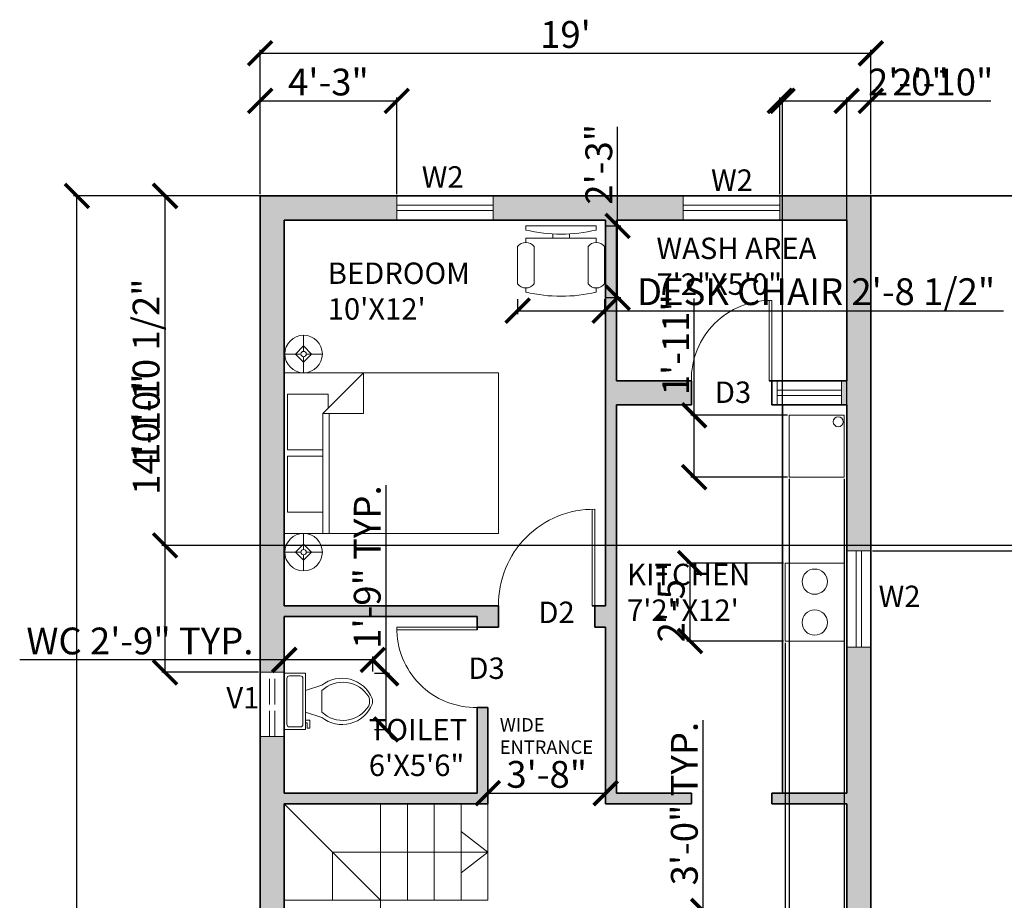
# Model space of a CAD drawing. Units: inches. Extents: x 2570 to 3313, y 1387 to 2106.
# Tile 3 of 5: x 2570 to 2938, y 1777 to 2106. Entities that reach past the tile are written whole.
import ezdxf

# ---------------------------------------------------------------- set-up
doc = ezdxf.new("R2010")
doc.units = ezdxf.units.IN
doc.linetypes.add('ACAD_ISO02W100', pattern=[15, 12, -3])
for name, color, linetype, lineweight in [('A-ANNO-DIMS', 7, 'Continuous', 18), ('A-ANNO-SYMB', 13, 'Continuous', 13), ('A-EQPM', 103, 'Continuous', 18), ('bed', 221, 'Continuous', 18), ('DOORS', 195, 'Continuous', 18), ('furniture', 11, 'Continuous', 18), ('KITCHEN', 103, 'Continuous', 25), ('P-FIXT', 8, 'Continuous', 18), ('STAIRS', 13, 'Continuous', 18), ('VENTILATORS', 143, 'ACAD_ISO02W100', 18), ('WALLS', 20, 'Continuous', 35), ('WINDOWS', 15, 'Continuous', 18)]:
    doc.layers.add(name, color=color, linetype=linetype, lineweight=lineweight)
for name, color, linetype, lineweight, true_color in [('A-ANNO-TEXT', 143, 'Continuous', 18, 0x7aafdf), ('A-AREA-IDEN', 143, 'Continuous', 18, 0x7aafdf), ('A-WALL-PATT', 30, 'Continuous', 13, 0xf26722)]:
    doc.layers.add(name, color=color, linetype=linetype, lineweight=lineweight, true_color=true_color)
doc.styles.get("Standard").update_dxf_attribs({"font": 'arial.ttf'})
doc.dimstyles.new('ISO-25', dxfattribs={"dimtxt": 10, "dimasz": 9, "dimexe": 1.25, "dimexo": 0.625, "dimtad": 1, "dimdec": 0, "dimlunit": 3, "dimtxsty": 'Standard', "dimblk": 'ARCHTICK', "dimcen": 2.5, "dimadec": 0, "dimazin": 0, "dimtfac": 1, "dimtdec": 0, "dimtmove": 0, "dimatfit": 3, "dimfxl": 1, "dimarcsym": 0})

# ---------------------------------------------------------------- blocks, each defined once
blk = doc.blocks.new('Lamp - Table')
for p, q in [((0, 7), (0, 1)), ((-1, 0), (-7, 0)), ((0, 3), (-3, 0)), ((-3, 0), (0, -3)), ((3, 0), (0, 3)), ((0, -3), (3, 0)), ((1, 0), (7, 0)), ((0, -1), (0, -7))]:
    blk.add_line(p, q)
for radius in [7, 1]:
    blk.add_circle((0, 0), radius)
blk = doc.blocks.new('Chair - Desk')
for p, q in [((-8.5, 0), (-8.5, -1)), ((-8.5, 0), (8.5, 0)), ((8.5, 0), (8.5, -1)), ((-2, -3), (-2, -1.9355)), ((2, -1.9576), (2, -3)), ((-8.5, -3), (-8.5, -4)), ((-8.5, -3), (8.5, -3)), ((8.5, -3), (8.5, -4)), ((-10.5, -5), (-10.5, -14)), ((-6.5, -14), (-6.5, -5)), ((6.5, -5), (6.5, -14)), ((10.5, -14), (10.5, -5)), ((-8.5, -15), (-8.5, -16)), ((8.5, -15), (8.5, -16))]:
    blk.add_line(p, q)
for centre, radius, start, end in [((0, 34.625), 36.625, 256.5803, 283.4197), ((-8.5, -6.5), 2.5, 36.8699, 143.1301), ((8.5, -6.5), 2.5, 36.8699, 143.1301), ((-8.5, -12.5), 2.5, 216.8699, 323.1301), ((8.5, -12.5), 2.5, 216.8699, 323.1301), ((0, 19.625), 36.625, 256.5803, 283.4197)]:
    blk.add_arc(centre, radius, start, end)
blk = doc.blocks.new('Toilet - top')
for p, q in [((9.5, -6), (9.5, -2)), ((-10, -8.5), (-8, -8.5)), ((-10, -9.5), (-10, -8.5)), ((-7, -9.5), (-10, -9.5)), ((-8, -8.5), (-8, -8)), ((-7, -8), (-7, -9.5)), ((-4, -8), (-6, -14)), ((4, -8), (6, -14)), ((4, -14), (-4, -14))]:
    blk.add_line(p, q)
blk.add_lwpolyline([(10.5, -8), (10.5, 0), (-10.5, 0), (-10.5, -8)], close=True)
for points in [[(-9.5, -2), (-9.5, -6)], [(8.5, -1), (-8.5, -1)], [(-8.5, -7), (8.5, -7)]]:
    blk.add_lwpolyline(points)
for centre, radius, start, end in [((-8.62, -1.88), 0.884, 81.8699, 188.1301), ((8.62, -1.88), 0.884, 351.8699, 98.1301), ((-8.62, -6.12), 0.884, 171.8699, 278.1301), ((8.62, -6.12), 0.884, 261.8699, 8.1301), ((3.52, -21.58), 12.17, 141.4691, 247.9714), ((4.2, -21.82), 11.33, 136.3677, 238.9468), ((-3.52, -21.58), 12.17, 292.0284, 38.5307), ((-4.2, -21.82), 11.33, 301.053, 43.6321), ((0, -27.88), 4, 245.7318, 294.2682), ((0, -29), 4, 254.8605, 285.1395)]:
    blk.add_arc(centre, radius, start, end)
blk = doc.blocks.new('Bed - Queen')
for p, q in [((0, -80.00003), (0, 0)), ((0, 0), (59.99999, 0)), ((59.99999, 0), (59.99999, -80.00003)), ((7.99999, -1.2), (28.79998, -1.2)), ((7.99999, -14.4), (7.99999, -1.2)), ((28.79998, -1.2), (28.79998, -14.4)), ((31.19999, -1.2), (51.99999, -1.2)), ((31.19999, -14.4), (31.19999, -1.2)), ((51.99999, -1.2), (51.99999, -16.4)), ((0, -14.4), (44.8, -14.4)), ((59.99999, -29.6), (44.8, -14.4)), ((44.8, -14.4), (44.8, -29.6)), ((44.8, -16.8), (0, -16.8)), ((51.99999, -16.4), (46.79936, -16.4)), ((44.8, -29.6), (59.99999, -29.6)), ((59.99999, -80.00003), (0, -80.00003))]:
    blk.add_line(p, q)
blk = doc.blocks.new('_ArchTick')
at = {"color": 0, "linetype": 'ByBlock', "const_width": 0.15}
blk.add_lwpolyline([(-0.5, -0.5), (0.5, 0.5)], dxfattribs=at)
blk = doc.blocks.new('*D20')
at = {"layer": 'A-ANNO-DIMS', "color": 0, "lineweight": -2, "transparency": 16777216}
for p, q in [((2659.53, 2040.49), (2590.49, 2040.49)), ((2591.74, 1440.49), (2591.74, 2040.49)), ((2659.53, 1440.49), (2590.49, 1440.49))]:
    blk.add_line(p, q, dxfattribs=at)
at = {"layer": 'Defpoints', "color": 0, "transparency": 16777216}
for p in [(2591.74, 2040.49), (2660.15, 2040.49), (2660.15, 1440.49)]:
    blk.add_point(p, dxfattribs=at)
at = {"layer": 'A-ANNO-DIMS', "color": 0, "lineweight": -2, "transparency": 16777216, "xscale": 9, "yscale": 9, "zscale": 9}
for p, rotation in [((2591.74, 2040.49), 90), ((2591.74, 1440.49), 270)]:
    blk.add_blockref('_ArchTick', p, dxfattribs=dict(at, rotation=rotation))
at = {"layer": 'A-ANNO-DIMS', "color": 0, "transparency": 16777216, "insert": (2586.01, 1740.49), "char_height": 10, "attachment_point": 5, "rotation": 90}
blk.add_mtext("50'", dxfattribs=at)
blk = doc.blocks.new('*D21')
at = {"layer": 'A-ANNO-DIMS', "color": 0, "lineweight": -2, "transparency": 16777216}
for p, q in [((2660.15, 2041.11), (2660.15, 2094.99)), ((2660.15, 2093.74), (2888.15, 2093.74)), ((2888.15, 2041.11), (2888.15, 2094.99))]:
    blk.add_line(p, q, dxfattribs=at)
at = {"layer": 'Defpoints', "color": 0, "transparency": 16777216}
for p in [(2888.15, 2093.74), (2660.15, 2040.49), (2888.15, 2040.49)]:
    blk.add_point(p, dxfattribs=at)
at = {"layer": 'A-ANNO-DIMS', "color": 0, "lineweight": -2, "transparency": 16777216, "xscale": 9, "yscale": 9, "zscale": 9, "rotation": 180}
blk.add_blockref('_ArchTick', (2660.15, 2093.74), dxfattribs=at)
at = {"layer": 'A-ANNO-DIMS', "color": 0, "lineweight": -2, "transparency": 16777216, "xscale": 9, "yscale": 9, "zscale": 9}
blk.add_blockref('_ArchTick', (2888.15, 2093.74), dxfattribs=at)
at = {"layer": 'A-ANNO-DIMS', "color": 0, "transparency": 16777216, "insert": (2774.15, 2099.47), "char_height": 10, "attachment_point": 5}
blk.add_mtext("19'", dxfattribs=at)
blk = doc.blocks.new('*D22')
at = {"layer": 'A-ANNO-DIMS', "color": 0, "lineweight": -2, "transparency": 16777216}
for p, q in [((2745.15, 1814.11), (2745.15, 1818.74)), ((2745.15, 1817.49), (2789.15, 1817.49)), ((2789.15, 1814.11), (2789.15, 1818.74))]:
    blk.add_line(p, q, dxfattribs=at)
at = {"layer": 'Defpoints', "color": 0, "transparency": 16777216}
for p in [(2789.15, 1817.49), (2745.15, 1813.49), (2789.15, 1813.49)]:
    blk.add_point(p, dxfattribs=at)
at = {"layer": 'A-ANNO-DIMS', "color": 0, "lineweight": -2, "transparency": 16777216, "xscale": 9, "yscale": 9, "zscale": 9, "rotation": 180}
blk.add_blockref('_ArchTick', (2745.15, 1817.49), dxfattribs=at)
at = {"layer": 'A-ANNO-DIMS', "color": 0, "lineweight": -2, "transparency": 16777216, "xscale": 9, "yscale": 9, "zscale": 9}
blk.add_blockref('_ArchTick', (2789.15, 1817.49), dxfattribs=at)
at = {"layer": 'A-ANNO-DIMS', "color": 0, "transparency": 16777216, "insert": (2767.15, 1823.22), "char_height": 10, "attachment_point": 5}
blk.add_mtext('3\'-8"', dxfattribs=at)
blk = doc.blocks.new('DOOR-SWING-30IN')
for p, q in [((0, 0), (-30, 0)), ((0, -1), (-30, -1))]:
    blk.add_line(p, q)
blk.add_arc((-0.5, -0.5), 29.5, 179.029, 270.971)
blk = doc.blocks.new('DOOR-SWING-36IN')
for p, q in [((-1, 0), (-1, 36)), ((0, 0), (0, 36))]:
    blk.add_line(p, q)
blk.add_arc((-0.5, 0.5), 35.5, 89.1931, 180.8069)
blk = doc.blocks.new('WIN-36IN')
for p, q in [((-36, 0), (-36, 9)), ((0, 0), (0, 9)), ((-36, 5.5), (0, 5.5)), ((-36, 3.5), (0, 3.5))]:
    blk.add_line(p, q)
blk = doc.blocks.new('VENT-V1-24IN')
for p, q in [((0, 0), (9, 0)), ((0, -24), (9, -24))]:
    blk.add_line(p, q)
at = {"ltscale": 0.8}
for p, q in [((3.5, -24), (3.5, 0)), ((5.5, -24), (5.5, 0))]:
    blk.add_line(p, q, dxfattribs=at)
blk = doc.blocks.new('*D47')
at = {"layer": 'A-ANNO-DIMS', "color": 0, "lineweight": -2, "transparency": 16777216}
for p, q in [((2669.15, 1862.9), (2669.15, 1868.48)), ((2702.2, 1862.9), (2702.2, 1868.48)), ((2669.15, 1867.23), (2570.38, 1867.23)), ((2702.2, 1867.23), (2669.15, 1867.23))]:
    blk.add_line(p, q, dxfattribs=at)
at = {"layer": 'Defpoints', "color": 0, "transparency": 16777216}
for p in [(2669.15, 1867.23), (2669.15, 1862.27), (2702.2, 1862.27)]:
    blk.add_point(p, dxfattribs=at)
at = {"layer": 'A-ANNO-DIMS', "color": 0, "lineweight": -2, "transparency": 16777216, "xscale": 9, "yscale": 9, "zscale": 9, "rotation": 180}
blk.add_blockref('_ArchTick', (2669.15, 1867.23), dxfattribs=at)
at = {"layer": 'A-ANNO-DIMS', "color": 0, "lineweight": -2, "transparency": 16777216, "xscale": 9, "yscale": 9, "zscale": 9}
blk.add_blockref('_ArchTick', (2702.2, 1867.23), dxfattribs=at)
at = {"layer": 'A-ANNO-DIMS', "color": 0, "transparency": 16777216, "insert": (2615.27, 1873.02), "char_height": 10, "attachment_point": 5}
blk.add_mtext('WC 2\'-9" TYP.', dxfattribs=at)
blk = doc.blocks.new('*D48')
at = {"layer": 'A-ANNO-DIMS', "color": 0, "lineweight": -2, "transparency": 16777216}
for p, q in [((2707.16, 1862.27), (2707.16, 1932.54)), ((2702.83, 1862.27), (2708.41, 1862.27)), ((2707.16, 1841.27), (2707.16, 1862.27)), ((2702.83, 1841.27), (2708.41, 1841.27))]:
    blk.add_line(p, q, dxfattribs=at)
at = {"layer": 'Defpoints', "color": 0, "transparency": 16777216}
for p in [(2702.2, 1862.27), (2707.16, 1862.27), (2702.2, 1841.27)]:
    blk.add_point(p, dxfattribs=at)
at = {"layer": 'A-ANNO-DIMS', "color": 0, "lineweight": -2, "transparency": 16777216, "xscale": 9, "yscale": 9, "zscale": 9}
for p, rotation in [((2707.16, 1862.27), 90), ((2707.16, 1841.27), 270)]:
    blk.add_blockref('_ArchTick', p, dxfattribs=dict(at, rotation=rotation))
at = {"layer": 'A-ANNO-DIMS', "color": 0, "transparency": 16777216, "insert": (2701.43, 1901.9), "char_height": 10, "attachment_point": 5, "rotation": 90}
blk.add_mtext('1\'-9" TYP.', dxfattribs=at)
blk = doc.blocks.new('*D54')
at = {"layer": 'A-ANNO-DIMS', "color": 0, "lineweight": -2, "transparency": 16777216}
for p, q in [((2825.55, 1773.49), (2825.55, 1844.69)), ((2805.78, 1773.49), (2826.8, 1773.49)), ((2825.55, 1737.49), (2825.55, 1773.49)), ((2805.78, 1737.49), (2826.8, 1737.49))]:
    blk.add_line(p, q, dxfattribs=at)
at = {"layer": 'Defpoints', "color": 0, "transparency": 16777216}
for p in [(2805.15, 1773.49), (2825.55, 1773.49), (2805.15, 1737.49)]:
    blk.add_point(p, dxfattribs=at)
at = {"layer": 'A-ANNO-DIMS', "color": 0, "lineweight": -2, "transparency": 16777216, "xscale": 9, "yscale": 9, "zscale": 9}
for p, rotation in [((2825.55, 1773.49), 90), ((2825.55, 1737.49), 270)]:
    blk.add_blockref('_ArchTick', p, dxfattribs=dict(at, rotation=rotation))
at = {"layer": 'A-ANNO-DIMS', "color": 0, "transparency": 16777216, "insert": (2819.82, 1813.59), "char_height": 10, "attachment_point": 5, "rotation": 90}
blk.add_mtext('3\'-0" TYP.', dxfattribs=at)
blk = doc.blocks.new('*D57')
at = {"layer": 'A-ANNO-DIMS', "color": 0, "lineweight": -2, "transparency": 16777216}
for p, q in [((2756.3, 2001.88), (2756.3, 1996.39)), ((2788.75, 2001.88), (2788.75, 1996.39)), ((2756.3, 1997.64), (2788.75, 1997.64)), ((2788.75, 1997.64), (2937.66, 1997.64))]:
    blk.add_line(p, q, dxfattribs=at)
at = {"layer": 'Defpoints', "color": 0, "transparency": 16777216}
for p in [(2756.3, 2002.51), (2788.75, 2002.51), (2788.75, 1997.64)]:
    blk.add_point(p, dxfattribs=at)
at = {"layer": 'A-ANNO-DIMS', "color": 0, "lineweight": -2, "transparency": 16777216, "xscale": 9, "yscale": 9, "zscale": 9, "rotation": 180}
blk.add_blockref('_ArchTick', (2756.3, 1997.64), dxfattribs=at)
at = {"layer": 'A-ANNO-DIMS', "color": 0, "lineweight": -2, "transparency": 16777216, "xscale": 9, "yscale": 9, "zscale": 9}
blk.add_blockref('_ArchTick', (2788.75, 1997.64), dxfattribs=at)
at = {"layer": 'A-ANNO-DIMS', "color": 0, "transparency": 16777216, "insert": (2867.7, 2003.44), "char_height": 10, "attachment_point": 5}
blk.add_mtext('DESK CHAIR 2\'-8 1/2"', dxfattribs=at)
blk = doc.blocks.new('*D58')
at = {"layer": 'A-ANNO-DIMS', "color": 0, "lineweight": -2, "transparency": 16777216}
for p, q in [((2793.62, 2029.3), (2793.62, 2066.3)), ((2789.38, 2029.3), (2794.87, 2029.3)), ((2793.62, 2002.51), (2793.62, 2029.3)), ((2789.38, 2002.51), (2794.87, 2002.51))]:
    blk.add_line(p, q, dxfattribs=at)
at = {"layer": 'Defpoints', "color": 0, "transparency": 16777216}
for p in [(2788.75, 2029.3), (2793.62, 2029.3), (2788.75, 2002.51)]:
    blk.add_point(p, dxfattribs=at)
at = {"layer": 'A-ANNO-DIMS', "color": 0, "lineweight": -2, "transparency": 16777216, "xscale": 9, "yscale": 9, "zscale": 9}
for p, rotation in [((2793.62, 2029.3), 90), ((2793.62, 2002.51), 270)]:
    blk.add_blockref('_ArchTick', p, dxfattribs=dict(at, rotation=rotation))
at = {"layer": 'A-ANNO-DIMS', "color": 0, "transparency": 16777216, "insert": (2787.88, 2052.3), "char_height": 10, "attachment_point": 5, "rotation": 90}
blk.add_mtext('2\'-3"', dxfattribs=at)
blk = doc.blocks.new('*D65')
at = {"layer": 'A-ANNO-DIMS', "color": 0, "lineweight": -2, "transparency": 16777216}
for p, q in [((2660.15, 2041.11), (2660.15, 2077.24)), ((2711.15, 2041.11), (2711.15, 2077.24)), ((2660.15, 2075.99), (2711.15, 2075.99))]:
    blk.add_line(p, q, dxfattribs=at)
at = {"layer": 'Defpoints', "color": 0, "transparency": 16777216}
for p in [(2711.15, 2075.99), (2660.15, 2040.49), (2711.15, 2040.49)]:
    blk.add_point(p, dxfattribs=at)
at = {"layer": 'A-ANNO-DIMS', "color": 0, "lineweight": -2, "transparency": 16777216, "xscale": 9, "yscale": 9, "zscale": 9, "rotation": 180}
blk.add_blockref('_ArchTick', (2660.15, 2075.99), dxfattribs=at)
at = {"layer": 'A-ANNO-DIMS', "color": 0, "lineweight": -2, "transparency": 16777216, "xscale": 9, "yscale": 9, "zscale": 9}
blk.add_blockref('_ArchTick', (2711.15, 2075.99), dxfattribs=at)
at = {"layer": 'A-ANNO-DIMS', "color": 0, "transparency": 16777216, "insert": (2685.65, 2081.72), "char_height": 10, "attachment_point": 5}
blk.add_mtext('4\'-3"', dxfattribs=at)
blk = doc.blocks.new('*D66')
at = {"layer": 'A-ANNO-DIMS', "color": 0, "lineweight": -2, "transparency": 16777216}
for p, q in [((2854.15, 2041.11), (2854.15, 2077.24)), ((2888.15, 2041.11), (2888.15, 2077.24)), ((2854.15, 2075.99), (2888.15, 2075.99)), ((2888.15, 2075.99), (2932.93, 2075.99))]:
    blk.add_line(p, q, dxfattribs=at)
at = {"layer": 'Defpoints', "color": 0, "transparency": 16777216}
for p in [(2888.15, 2075.99), (2854.15, 2040.49), (2888.15, 2040.49)]:
    blk.add_point(p, dxfattribs=at)
at = {"layer": 'A-ANNO-DIMS', "color": 0, "lineweight": -2, "transparency": 16777216, "xscale": 9, "yscale": 9, "zscale": 9, "rotation": 180}
blk.add_blockref('_ArchTick', (2854.15, 2075.99), dxfattribs=at)
at = {"layer": 'A-ANNO-DIMS', "color": 0, "lineweight": -2, "transparency": 16777216, "xscale": 9, "yscale": 9, "zscale": 9}
blk.add_blockref('_ArchTick', (2888.15, 2075.99), dxfattribs=at)
at = {"layer": 'A-ANNO-DIMS', "color": 0, "transparency": 16777216, "insert": (2915.04, 2081.72), "char_height": 10, "attachment_point": 5}
blk.add_mtext('2\'-10"', dxfattribs=at)
blk = doc.blocks.new('*D67')
at = {"layer": 'A-ANNO-DIMS', "color": 0, "lineweight": -2, "transparency": 16777216}
for p, q in [((2888.78, 2040.49), (3222.91, 2040.49)), ((3221.66, 1907.99), (3221.66, 2040.49)), ((2888.78, 1907.99), (3222.91, 1907.99))]:
    blk.add_line(p, q, dxfattribs=at)
at = {"layer": 'Defpoints', "color": 0, "transparency": 16777216}
for p in [(2888.15, 2040.49), (3221.66, 2040.49), (2888.15, 1907.99)]:
    blk.add_point(p, dxfattribs=at)
at = {"layer": 'A-ANNO-DIMS', "color": 0, "lineweight": -2, "transparency": 16777216, "xscale": 9, "yscale": 9, "zscale": 9}
for p, rotation in [((3221.66, 2040.49), 90), ((3221.66, 1907.99), 270)]:
    blk.add_blockref('_ArchTick', p, dxfattribs=dict(at, rotation=rotation))
at = {"layer": 'A-ANNO-DIMS', "color": 0, "transparency": 16777216, "insert": (3215.87, 1974.24), "char_height": 10, "attachment_point": 5, "rotation": 90}
blk.add_mtext('11\'-0 1/2"', dxfattribs=at)
blk = doc.blocks.new('*D70')
at = {"layer": 'A-ANNO-DIMS', "color": 0, "lineweight": -2, "transparency": 16777216}
for p, q in [((2957.54, 2040.49), (2623.4, 2040.49)), ((2624.65, 1909.99), (2624.65, 2040.49)), ((2957.54, 1909.99), (2623.4, 1909.99))]:
    blk.add_line(p, q, dxfattribs=at)
at = {"layer": 'Defpoints', "color": 0, "transparency": 16777216}
for p in [(2624.65, 2040.49), (2958.16, 2040.49), (2958.16, 1909.99)]:
    blk.add_point(p, dxfattribs=at)
at = {"layer": 'A-ANNO-DIMS', "color": 0, "lineweight": -2, "transparency": 16777216, "xscale": 9, "yscale": 9, "zscale": 9}
for p, rotation in [((2624.65, 2040.49), 90), ((2624.65, 1909.99), 270)]:
    blk.add_blockref('_ArchTick', p, dxfattribs=dict(at, rotation=rotation))
at = {"layer": 'A-ANNO-DIMS', "color": 0, "transparency": 16777216, "insert": (2618.86, 1975.24), "char_height": 10, "attachment_point": 5, "rotation": 90}
blk.add_mtext('10\'-10 1/2"', dxfattribs=at)
blk = doc.blocks.new('*D75')
at = {"layer": 'A-ANNO-DIMS', "color": 0, "lineweight": -2, "transparency": 16777216}
for p, q in [((2659.53, 2040.49), (2623.4, 2040.49)), ((2624.65, 1862.62), (2624.65, 2040.49)), ((2659.53, 1862.62), (2623.4, 1862.62))]:
    blk.add_line(p, q, dxfattribs=at)
at = {"layer": 'Defpoints', "color": 0, "transparency": 16777216}
for p in [(2624.65, 2040.49), (2660.15, 2040.49), (2660.15, 1862.62)]:
    blk.add_point(p, dxfattribs=at)
at = {"layer": 'A-ANNO-DIMS', "color": 0, "lineweight": -2, "transparency": 16777216, "xscale": 9, "yscale": 9, "zscale": 9}
for p, rotation in [((2624.65, 2040.49), 90), ((2624.65, 1862.62), 270)]:
    blk.add_blockref('_ArchTick', p, dxfattribs=dict(at, rotation=rotation))
at = {"layer": 'A-ANNO-DIMS', "color": 0, "transparency": 16777216, "insert": (2618.92, 1951.55), "char_height": 10, "attachment_point": 5, "rotation": 90}
blk.add_mtext('14\'-10"', dxfattribs=at)
blk = doc.blocks.new('*D80')
at = {"layer": 'A-ANNO-DIMS', "color": 0, "lineweight": -2, "transparency": 16777216}
for p, q in [((2855.15, 1818.11), (2855.15, 2077.24)), ((2879.15, 1818.11), (2879.15, 2077.24)), ((2855.15, 2075.99), (2879.15, 2075.99)), ((2879.15, 2075.99), (2916.16, 2075.99))]:
    blk.add_line(p, q, dxfattribs=at)
at = {"layer": 'Defpoints', "color": 0, "transparency": 16777216}
for p in [(2879.15, 2075.99), (2855.15, 1817.49), (2879.15, 1817.49)]:
    blk.add_point(p, dxfattribs=at)
at = {"layer": 'A-ANNO-DIMS', "color": 0, "lineweight": -2, "transparency": 16777216, "xscale": 9, "yscale": 9, "zscale": 9, "rotation": 180}
blk.add_blockref('_ArchTick', (2855.15, 2075.99), dxfattribs=at)
at = {"layer": 'A-ANNO-DIMS', "color": 0, "lineweight": -2, "transparency": 16777216, "xscale": 9, "yscale": 9, "zscale": 9}
blk.add_blockref('_ArchTick', (2879.15, 2075.99), dxfattribs=at)
at = {"layer": 'A-ANNO-DIMS', "color": 0, "transparency": 16777216, "insert": (2902.16, 2081.72), "char_height": 10, "attachment_point": 5}
blk.add_mtext('2\'-0"', dxfattribs=at)
blk = doc.blocks.new('*D81')
at = {"layer": 'A-ANNO-DIMS', "color": 0, "lineweight": -2, "transparency": 16777216}
for p, q in [((2856.15, 1873.66), (2856.15, 1403.74)), ((2878.15, 1873.66), (2878.15, 1403.74)), ((2856.15, 1404.99), (2878.15, 1404.99)), ((2878.15, 1404.99), (2921.82, 1404.99))]:
    blk.add_line(p, q, dxfattribs=at)
at = {"layer": 'Defpoints', "color": 0, "transparency": 16777216}
for p in [(2856.15, 1874.28), (2878.15, 1874.28), (2878.15, 1404.99)]:
    blk.add_point(p, dxfattribs=at)
at = {"layer": 'A-ANNO-DIMS', "color": 0, "lineweight": -2, "transparency": 16777216, "xscale": 9, "yscale": 9, "zscale": 9, "rotation": 180}
blk.add_blockref('_ArchTick', (2856.15, 1404.99), dxfattribs=at)
at = {"layer": 'A-ANNO-DIMS', "color": 0, "lineweight": -2, "transparency": 16777216, "xscale": 9, "yscale": 9, "zscale": 9}
blk.add_blockref('_ArchTick', (2878.15, 1404.99), dxfattribs=at)
at = {"layer": 'A-ANNO-DIMS', "color": 0, "transparency": 16777216, "insert": (2904.48, 1410.72), "char_height": 10, "attachment_point": 5}
blk.add_mtext('1\'-10"', dxfattribs=at)
blk = doc.blocks.new('*D82')
at = {"layer": 'A-ANNO-DIMS', "color": 0, "lineweight": -2, "transparency": 16777216}
for p, q in [((2855.53, 1903.39), (2819.4, 1903.39)), ((2820.65, 1874.28), (2820.65, 1903.39)), ((2855.53, 1874.28), (2819.4, 1874.28))]:
    blk.add_line(p, q, dxfattribs=at)
at = {"layer": 'Defpoints', "color": 0, "transparency": 16777216}
for p in [(2820.65, 1903.39), (2856.15, 1903.39), (2856.15, 1874.28)]:
    blk.add_point(p, dxfattribs=at)
at = {"layer": 'A-ANNO-DIMS', "color": 0, "lineweight": -2, "transparency": 16777216, "xscale": 9, "yscale": 9, "zscale": 9}
for p, rotation in [((2820.65, 1903.39), 90), ((2820.65, 1874.28), 270)]:
    blk.add_blockref('_ArchTick', p, dxfattribs=dict(at, rotation=rotation))
at = {"layer": 'A-ANNO-DIMS', "color": 0, "transparency": 16777216, "insert": (2814.92, 1888.84), "char_height": 10, "attachment_point": 5, "rotation": 90}
blk.add_mtext('2\'-5"', dxfattribs=at)
blk = doc.blocks.new('*D83')
at = {"layer": 'A-ANNO-DIMS', "color": 0, "lineweight": -2, "transparency": 16777216}
for p, q in [((2857.69, 1934.86), (2857.69, 1403.74)), ((2878.15, 1934.86), (2878.15, 1403.74)), ((2857.69, 1404.99), (2878.15, 1404.99)), ((2878.15, 1404.99), (2937.35, 1404.99))]:
    blk.add_line(p, q, dxfattribs=at)
at = {"layer": 'Defpoints', "color": 0, "transparency": 16777216}
for p in [(2857.69, 1935.48), (2878.15, 1935.48), (2878.15, 1404.99)]:
    blk.add_point(p, dxfattribs=at)
at = {"layer": 'A-ANNO-DIMS', "color": 0, "lineweight": -2, "transparency": 16777216, "xscale": 9, "yscale": 9, "zscale": 9, "rotation": 180}
blk.add_blockref('_ArchTick', (2857.69, 1404.99), dxfattribs=at)
at = {"layer": 'A-ANNO-DIMS', "color": 0, "lineweight": -2, "transparency": 16777216, "xscale": 9, "yscale": 9, "zscale": 9}
blk.add_blockref('_ArchTick', (2878.15, 1404.99), dxfattribs=at)
at = {"layer": 'A-ANNO-DIMS', "color": 0, "transparency": 16777216, "insert": (2912.25, 1410.78), "char_height": 10, "attachment_point": 5}
blk.add_mtext('1\'-8 1/2"', dxfattribs=at)
blk = doc.blocks.new('*D84')
at = {"layer": 'A-ANNO-DIMS', "color": 0, "lineweight": -2, "transparency": 16777216}
for p, q in [((2822.19, 1958.58), (2822.19, 2002.24)), ((2857.07, 1958.58), (2820.94, 1958.58)), ((2822.19, 1935.48), (2822.19, 1958.58)), ((2857.07, 1935.48), (2820.94, 1935.48))]:
    blk.add_line(p, q, dxfattribs=at)
at = {"layer": 'Defpoints', "color": 0, "transparency": 16777216}
for p in [(2822.19, 1958.58), (2857.69, 1958.58), (2857.69, 1935.48)]:
    blk.add_point(p, dxfattribs=at)
at = {"layer": 'A-ANNO-DIMS', "color": 0, "lineweight": -2, "transparency": 16777216, "xscale": 9, "yscale": 9, "zscale": 9}
for p, rotation in [((2822.19, 1958.58), 90), ((2822.19, 1935.48), 270)]:
    blk.add_blockref('_ArchTick', p, dxfattribs=dict(at, rotation=rotation))
at = {"layer": 'A-ANNO-DIMS', "color": 0, "transparency": 16777216, "insert": (2816.55, 1984.91), "char_height": 10, "attachment_point": 5, "rotation": 90}
blk.add_mtext('1\'-11"', dxfattribs=at)

msp = doc.modelspace()

# ---------------------------------------------------------------- hatches: boundary and pattern name
at = {"layer": 'A-WALL-PATT'}
h = msp.add_hatch(color=256, dxfattribs=at)
h.dxf.hatch_style = 1
h.paths.add_polyline_path([(2888.15, 1871.99), (2879.15, 1871.99), (2879.15, 1817.49), (2851.15, 1817.49), (2851.15, 1813.49), (2879.15, 1813.49), (2879.15, 1657.4), (2888.15, 1657.4)])
h.paths.add_polyline_path([(2831.15, 1737.49), (2669.15, 1737.49), (2669.15, 1813.49), (2745.15, 1813.49), (2745.15, 1849.49), (2741.15, 1849.49), (2741.15, 1817.49), (2669.15, 1817.49), (2669.15, 1838.62), (2660.15, 1838.62), (2660.15, 1669.99), (2669.15, 1669.99), (2669.15, 1728.49), (2831.15, 1728.49)])
h.paths.add_polyline_path([(2669.15, 1621.99), (2660.15, 1621.99), (2660.15, 1440.49), (2802.65, 1440.49), (2802.65, 1449.49), (2669.15, 1449.49), (2669.15, 1554.49), (2700.9, 1554.49), (2700.9, 1563.49), (2669.15, 1563.49)])
h.paths.add_polyline_path([(2780.65, 1563.49), (2748.9, 1563.49), (2748.9, 1554.49), (2780.65, 1554.49)], flags=17)
h.paths.add_polyline_path([(2836.15, 1599.49), (2879.15, 1599.49), (2879.15, 1449.49), (2874.65, 1449.49), (2874.65, 1440.49), (2888.15, 1440.49), (2888.15, 1633.4), (2879.15, 1633.4), (2879.15, 1608.49), (2831.15, 1608.49), (2831.15, 1680.49), (2827.15, 1680.49), (2827.15, 1563.49), (2822.65, 1563.49), (2822.65, 1554.49), (2836.15, 1554.49)])
h.paths.add_polyline_path([(2793.15, 1962.49), (2821.15, 1962.49), (2821.15, 1971.49), (2793.15, 1971.49), (2793.15, 2031.49), (2818.15, 2031.49), (2818.15, 2040.49), (2747.15, 2040.49), (2747.15, 2031.49), (2789.15, 2031.49), (2789.15, 1887.49), (2785.15, 1887.49), (2785.15, 1879.49), (2789.15, 1879.49), (2789.15, 1817.49), (2789.15, 1813.49), (2793.15, 1813.49), (2821.15, 1813.49), (2821.15, 1817.49), (2793.15, 1817.49)])
h.paths.add_polyline_path([(2749.15, 1887.49), (2669.15, 1887.49), (2669.15, 2031.49), (2711.15, 2031.49), (2711.15, 2040.49), (2660.15, 2040.49), (2660.15, 1862.62), (2669.15, 1862.62), (2669.15, 1883.49), (2741.15, 1883.49), (2741.15, 1879.49), (2749.15, 1879.49)])
h.paths.add_polyline_path([(2888.15, 2040.49), (2854.15, 2040.49), (2854.15, 2031.49), (2879.15, 2031.49), (2879.15, 1971.49), (2877.15, 1971.49), (2877.15, 1962.49), (2879.15, 1962.49), (2879.15, 1907.99), (2888.15, 1907.99)])
h.paths.add_polyline_path([(2967.16, 2031.49), (3011.16, 2031.49), (3011.16, 2004.49), (3015.16, 2004.49), (3015.16, 2031.49), (3039.26, 2031.49), (3039.26, 2040.49), (2958.16, 2040.49), (2958.16, 1909.99), (2967.16, 1909.99), (2967.16, 1921.99), (2967.16, 1966.49)])
h.paths.add_polyline_path([(3186.16, 2040.49), (3063.26, 2040.49), (3063.26, 2031.49), (3087.16, 2031.49), (3087.16, 1970.49), (3015.16, 1970.49), (3015.16, 1974.49), (3011.16, 1974.49), (3011.16, 1966.49), (3177.16, 1966.49), (3177.16, 1817.49), (3172.66, 1817.49), (3172.66, 1813.49), (3177.16, 1813.49), (3177.16, 1721.56), (3186.16, 1721.56)])
h.paths.add_polyline_path([(3177.16, 2031.49), (3177.16, 1970.49), (3091.16, 1970.49), (3091.16, 2031.49)], flags=16)
h.paths.add_polyline_path([(2967.16, 1873.99), (2958.16, 1873.99), (2958.16, 1712.62), (2967.16, 1712.62), (2967.16, 1724.49), (3051.16, 1724.49), (3051.16, 1710.49), (3055.16, 1710.49), (3055.16, 1724.49), (3125.16, 1724.49), (3125.16, 1676.49), (3085.16, 1676.49), (3085.16, 1672.49), (3125.16, 1672.49), (3125.16, 1668.49), (3129.16, 1668.49), (3129.16, 1733.49), (2967.16, 1733.49), (2967.16, 1813.49), (3136.66, 1813.49), (3136.66, 1817.49), (2967.16, 1817.49)])
h.paths.add_polyline_path([(2967.16, 1672.49), (3055.16, 1672.49), (3055.16, 1680.49), (3051.16, 1680.49), (3051.16, 1676.49), (2967.16, 1676.49), (2967.16, 1688.62), (2958.16, 1688.62), (2958.16, 1618.49), (2967.16, 1618.49), (2967.16, 1631.69)])
h.paths.add_polyline_path([(3186.16, 1685.56), (3177.16, 1685.56), (3177.16, 1568.09), (3169.16, 1568.09), (3169.16, 1564.09), (3177.16, 1564.09), (3177.16, 1519.49), (3177.16, 1449.49), (3186.16, 1449.49)])
h.paths.add_polyline_path([(3129.16, 1564.09), (3129.16, 1632.49), (3125.16, 1632.49), (3125.16, 1528.49), (2967.16, 1528.49), (2967.16, 1582.49), (2958.16, 1582.49), (2958.16, 1449.49), (2967.16, 1449.49), (2967.16, 1519.49), (3129.16, 1519.49)])
h.paths.add_polyline_path([(3123.16, 1975.63), (3150.13, 1975.63), (3150.13, 1992.12), (3123.16, 1992.12)], flags=8)
h.paths.add_polyline_path([(3130.18, 1590.82), (3180.42, 1590.82), (3180.42, 1617.03), (3130.18, 1617.03)], flags=9)

# ---------------------------------------------------------------- linework, layer by layer
at = {"layer": 'A-ANNO-SYMB'}
for p, q in [((2745.15, 1795.49), (2735.15, 1803.19)), ((2687.15, 1777.49), (2687.15, 1795.49)), ((2687.15, 1795.49), (2745.15, 1795.49)), ((2745.15, 1795.49), (2735.15, 1787.79))]:
    msp.add_line(p, q, dxfattribs=at)
at = {"layer": 'A-EQPM'}
for p, q in [((2856.15, 1903.39), (2856.15, 1874.28)), ((2878.15, 1903.39), (2856.15, 1903.39)), ((2878.15, 1903.39), (2878.15, 1874.28)), ((2878.15, 1874.28), (2856.15, 1874.28))]:
    msp.add_line(p, q, dxfattribs=at)
for centre in [(2867.21, 1896.47), (2867.21, 1881.2)]:
    msp.add_circle(centre, 4.72, dxfattribs=at)
at = {"layer": 'KITCHEN'}
msp.add_line((2855.15, 1962.49), (2855.15, 1817.49), dxfattribs=at)
at = {"layer": 'P-FIXT'}
for p, q in [((2857.69, 1935.48), (2857.69, 1958.58)), ((2857.69, 1958.58), (2878.15, 1958.58)), ((2878.15, 1958.58), (2878.15, 1935.48)), ((2878.15, 1935.48), (2857.69, 1935.48))]:
    msp.add_line(p, q, dxfattribs=at)
msp.add_circle((2875.97, 1956.16), 1.86, dxfattribs=at)
at = {"layer": 'STAIRS'}
for p, q in [((2705.15, 1777.49), (2669.15, 1813.49)), ((2705.15, 1777.49), (2705.15, 1813.49)), ((2715.15, 1777.49), (2715.15, 1813.49)), ((2725.15, 1777.49), (2725.15, 1813.49)), ((2735.15, 1777.49), (2735.15, 1813.49)), ((2745.15, 1777.49), (2745.15, 1813.49)), ((2669.15, 1777.49), (2745.15, 1777.49)), ((2705.15, 1773.49), (2705.15, 1777.49))]:
    msp.add_line(p, q, dxfattribs=at)
at = {"layer": 'WALLS'}
for p, q in [((2660.15, 2040.49), (2888.15, 2040.49)), ((2660.15, 1440.49), (2660.15, 2040.49)), ((2888.15, 2040.49), (2888.15, 1440.49)), ((2669.15, 2031.49), (2789.15, 2031.49)), ((2669.15, 1887.49), (2669.15, 2031.49)), ((2789.15, 1887.49), (2789.15, 2031.49)), ((2793.15, 2031.49), (2879.15, 2031.49)), ((2793.15, 1971.49), (2793.15, 2031.49)), ((2879.15, 2031.49), (2879.15, 1971.49)), ((2793.15, 1971.49), (2821.15, 1971.49)), ((2821.15, 1962.49), (2821.15, 1971.49)), ((2850.15, 1971.49), (2879.15, 1971.49)), ((2851.15, 1962.49), (2851.15, 1971.49)), ((2793.15, 1817.49), (2793.15, 1962.49)), ((2793.15, 1962.49), (2821.15, 1962.49)), ((2851.15, 1962.49), (2879.15, 1962.49)), ((2879.15, 1962.49), (2879.15, 1817.49)), ((2669.15, 1887.49), (2749.15, 1887.49)), ((2749.15, 1887.49), (2749.15, 1879.49)), ((2784.15, 1887.49), (2789.15, 1887.49)), ((2785.15, 1887.49), (2785.15, 1879.49)), ((2669.15, 1883.49), (2741.15, 1883.49)), ((2669.15, 1817.49), (2669.15, 1883.49)), ((2741.15, 1878.49), (2741.15, 1883.49)), ((2741.15, 1879.49), (2749.15, 1879.49)), ((2785.15, 1879.49), (2789.15, 1879.49)), ((2789.15, 1817.49), (2789.15, 1879.49)), ((2741.15, 1817.49), (2741.15, 1849.49)), ((2741.15, 1849.49), (2745.15, 1849.49)), ((2745.15, 1813.49), (2745.15, 1849.49)), ((2669.15, 1817.49), (2741.15, 1817.49)), ((2789.15, 1813.49), (2789.15, 1817.49)), ((2793.15, 1817.49), (2821.15, 1817.49)), ((2821.15, 1817.49), (2821.15, 1813.49)), ((2851.15, 1817.49), (2851.15, 1813.49)), ((2851.15, 1817.49), (2879.15, 1817.49)), ((2669.15, 1813.49), (2745.15, 1813.49)), ((2669.15, 1737.49), (2669.15, 1813.49)), ((2789.15, 1813.49), (2793.15, 1813.49)), ((2789.15, 1813.49), (2821.15, 1813.49)), ((2851.15, 1813.49), (2879.15, 1813.49)), ((2879.15, 1813.49), (2879.15, 1608.49))]:
    msp.add_line(p, q, dxfattribs=at)
at = {"layer": 'WINDOWS'}
for p, q in [((2853.15, 1962.49), (2853.15, 1971.49)), ((2877.15, 1962.49), (2877.15, 1971.49)), ((2877.15, 1967.99), (2853.15, 1967.99)), ((2877.15, 1965.99), (2853.15, 1965.99))]:
    msp.add_line(p, q, dxfattribs=at)

# ---------------------------------------------------------------- block references
at = {"layer": 'bed', "xscale": -1, "rotation": 180}
msp.add_blockref('Lamp - Table', (2676.38, 1981.46), dxfattribs=at)
at = {"layer": 'bed', "rotation": 90}
msp.add_blockref('Bed - Queen', (2669.15, 1914.47), dxfattribs=at)
at = {"layer": 'bed'}
msp.add_blockref('Lamp - Table', (2676.38, 1907.47), dxfattribs=at)
at = {"layer": 'DOORS', "rotation": 269.9999999999988}
msp.add_blockref('DOOR-SWING-30IN', (2851.15, 1971.49), dxfattribs=at)
at = {"layer": 'DOORS'}
for name, p in [('DOOR-SWING-36IN', (2785.15, 1887.49)), ('DOOR-SWING-30IN', (2741.15, 1879.49))]:
    msp.add_blockref(name, p, dxfattribs=at)
at = {"layer": 'furniture', "xscale": 1.545430965225023, "yscale": 1.545430965225023, "zscale": 1.545430965225023}
msp.add_blockref('Chair - Desk', (2772.52, 2029.3), dxfattribs=at)
at = {"layer": 'P-FIXT', "rotation": 90}
msp.add_blockref('Toilet - top', (2669.15, 1851.77), dxfattribs=at)
at = {"layer": 'VENTILATORS'}
msp.add_blockref('VENT-V1-24IN', (2660.15, 1862.62), dxfattribs=at)
at = {"layer": 'WINDOWS'}
msp.add_blockref('WIN-36IN', (2747.15, 2031.49), dxfattribs=at)
for p, rotation in [((2818.15, 2040.49), 180), ((2888.15, 1907.99), 90.00000000000239)]:
    msp.add_blockref('WIN-36IN', p, dxfattribs=dict(at, rotation=rotation))

# ---------------------------------------------------------------- texts
at = {"layer": 'A-ANNO-TEXT', "char_height": 8, "attachment_point": 1}
for s, width, insert in [('W2', 13.4987, (2720.49, 2051.57)), ('W2', 13.4987, (2828.5, 2050.38)), ('D3', 13.0839, (2829.92, 1971.19)), ('W2', 13.4987, (2891.06, 1894.97)), ('D2', 13.0839, (2764.02, 1889)), ('D3', 13.0839, (2737.9, 1868.14)), ('V1', 13.4987, (2647.53, 1857.12))]:
    msp.add_mtext_dynamic_manual_height_columns(s, width=width, gutter_width=12.5, heights=[0], dxfattribs=dict(at, insert=insert))
at = {"layer": 'A-AREA-IDEN', "attachment_point": 1}
for s, width, insert, char_height in [('WASH AREA\\P7\'2"X5\'0"', 89.0594, (2808.11, 2024.89), 8), ("BEDROOM\\P10'X12'", 60.8198, (2685.39, 2015.62), 8), ('KITCHEN\\P7\'2"X12\'', 60.8198, (2797.14, 1903.14), 8), ('TOILET\\P6\'X5\'6"', 60.8198, (2700.72, 1845.22), 8), ('WIDE ENTRANCE', 37.3943, (2749.64, 1845.51), 5)]:
    msp.add_mtext_dynamic_manual_height_columns(s, width=width, gutter_width=12.5, heights=[0], dxfattribs=dict(at, insert=insert, char_height=char_height))

# ---------------------------------------------------------------- dimensions: what is measured, and where the dimension line sits
at = {"layer": 'A-ANNO-DIMS'}
for base, p1, p2, override, picture, middle in [((2888.15, 2093.74), (2660.15, 2040.49), (2888.15, 2040.49), {"dimclrd": 0, "dimclre": 0, "dimclrt": 0}, '*D21', (2774.15, 2099.47)), ((2711.15, 2075.99), (2660.15, 2040.49), (2711.15, 2040.49), {"dimdec": 1, "dimlfac": 1, "dimrnd": 0, "dimzin": 1, "dimdsep": 46, "dimlunit": 4, "dimfrac": 2}, '*D65', (2685.65, 2081.72)), ((2888.15, 2075.99), (2854.15, 2040.49), (2888.15, 2040.49), {"dimdec": 1, "dimlfac": 1, "dimrnd": 0, "dimzin": 1, "dimdsep": 46, "dimlunit": 4, "dimfrac": 2}, '*D66', (2915.04, 2081.72)), ((2879.15, 2075.99), (2855.15, 1817.49), (2879.15, 1817.49), {"dimdec": 1, "dimlfac": 1, "dimrnd": 0, "dimzin": 1, "dimdsep": 46, "dimlunit": 4, "dimfrac": 2}, '*D80', (2902.16, 2081.72)), ((2878.15, 1404.99), (2857.69, 1935.48), (2878.15, 1935.48), {"dimdec": 1, "dimlfac": 1, "dimrnd": 0, "dimzin": 1, "dimdsep": 46, "dimlunit": 4, "dimfrac": 2}, '*D83', (2912.25, 1410.78)), ((2878.15, 1404.99), (2856.15, 1874.28), (2878.15, 1874.28), {"dimdec": 1, "dimlfac": 1, "dimrnd": 0, "dimzin": 1, "dimdsep": 46, "dimlunit": 4, "dimfrac": 2}, '*D81', (2904.48, 1410.72)), ((2789.15, 1817.49), (2745.15, 1813.49), (2789.15, 1813.49), {"dimclrd": 0, "dimclre": 0, "dimclrt": 0}, '*D22', (2767.15, 1823.22))]:
    dim = msp.add_linear_dim(base=base, p1=p1, p2=p2, dimstyle='ISO-25', override=override, dxfattribs=at)
    dim.commit()
    dim.dimension.update_dxf_attribs({"geometry": picture, "text_midpoint": middle})
for base, p1, p2, override, picture, middle in [((2793.62, 2029.3), (2788.75, 2002.51), (2788.75, 2029.3), {"dimdec": 1, "dimlfac": 1, "dimrnd": 0, "dimzin": 1, "dimdsep": 46, "dimlunit": 4, "dimfrac": 2}, '*D58', (2787.88, 2052.3)), ((2591.74, 2040.49), (2660.15, 1440.49), (2660.15, 2040.49), {"dimclrd": 0, "dimclre": 0, "dimclrt": 0}, '*D20', (2586.01, 1740.49)), ((2624.65, 2040.49), (2958.16, 1909.99), (2958.16, 2040.49), {"dimdec": 1, "dimlfac": 1, "dimrnd": 0, "dimzin": 1, "dimdsep": 46, "dimlunit": 4, "dimfrac": 2}, '*D70', (2618.86, 1975.24)), ((2624.65, 2040.49), (2660.15, 1862.62), (2660.15, 2040.49), {"dimdec": 1, "dimlfac": 1, "dimrnd": 0, "dimzin": 1, "dimdsep": 46, "dimlunit": 4, "dimfrac": 2}, '*D75', (2618.92, 1951.55)), ((3221.66, 2040.49), (2888.15, 1907.99), (2888.15, 2040.49), {"dimdec": 1, "dimlfac": 1, "dimrnd": 0, "dimzin": 1, "dimdsep": 46, "dimlunit": 4, "dimfrac": 2}, '*D67', (3215.87, 1974.24)), ((2822.19, 1958.58), (2857.69, 1935.48), (2857.69, 1958.58), {"dimdec": 1, "dimlfac": 1, "dimrnd": 0, "dimzin": 1, "dimdsep": 46, "dimlunit": 4, "dimfrac": 2}, '*D84', (2816.55, 1984.91)), ((2820.65, 1903.39), (2856.15, 1874.28), (2856.15, 1903.39), {"dimdec": 1, "dimlfac": 1, "dimrnd": 0, "dimzin": 1, "dimdsep": 46, "dimlunit": 4, "dimfrac": 2}, '*D82', (2814.92, 1888.84))]:
    dim = msp.add_linear_dim(base=base, p1=p1, p2=p2, angle=90, dimstyle='ISO-25', override=override, dxfattribs=at)
    dim.commit()
    dim.dimension.update_dxf_attribs({"geometry": picture, "text_midpoint": middle})
dim = msp.add_linear_dim(base=(2788.7508, 1997.6398), p1=(2756.2968, 2002.508), p2=(2788.7508, 2002.508), text='DESK CHAIR <>', dimstyle='ISO-25', override={"dimdec": 1, "dimlfac": 1, "dimrnd": 0, "dimzin": 1, "dimdsep": 46, "dimlunit": 4, "dimfrac": 2}, dxfattribs=at)
dim.commit()
dim.dimension.update_dxf_attribs({"geometry": '*D57', "text_midpoint": (2867.7039, 2003.4354)})
for base, p1, p2, angle, text, picture, middle in [((2707.16, 1862.27), (2702.2, 1841.27), (2702.2, 1862.27), 90, '<> TYP.', '*D48', (2701.43, 1901.9)), ((2669.1545, 1867.2293), (2702.2008, 1862.2724), (2669.1545, 1862.2724), 180, 'WC <> TYP.', '*D47', (2615.2697, 1873.0248)), ((2825.55, 1773.49), (2805.15, 1737.49), (2805.15, 1773.49), 90, '<> TYP.', '*D54', (2819.82, 1813.59))]:
    dim = msp.add_linear_dim(base=base, p1=p1, p2=p2, angle=angle, text=text, dimstyle='ISO-25', override={"dimdec": 1, "dimlfac": 1, "dimrnd": 0, "dimzin": 1, "dimdsep": 46, "dimlunit": 4, "dimfrac": 2}, dxfattribs=at)
    dim.commit()
    dim.dimension.update_dxf_attribs({"geometry": picture, "text_midpoint": middle})

doc.saveas('drawing.dxf')
